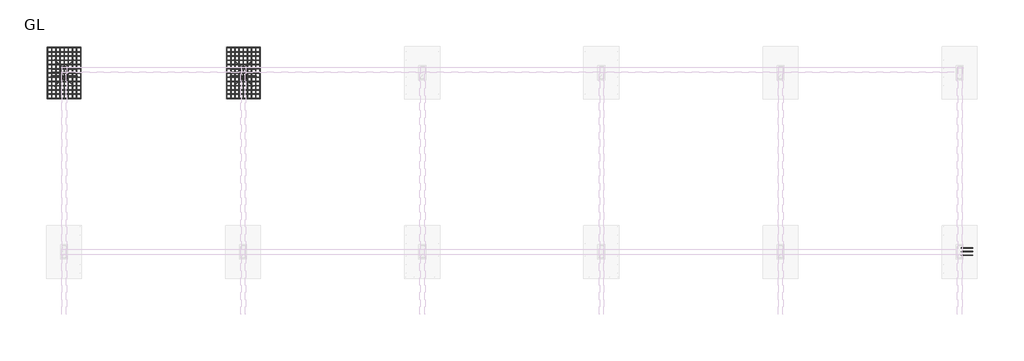
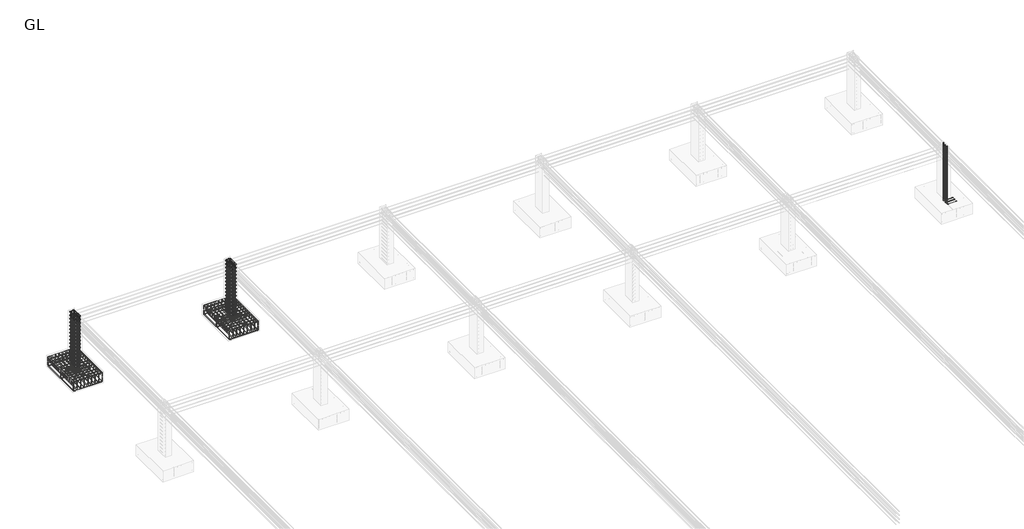
# One storey, part 14 of 16: 23 reinforcing bars.
"""IFC4 building model written with IfcOpenShell, lengths in millimetres."""

from ifc_helpers import new_model, si_unit, point, frame, origin, place, context, project, spatial, polyline, circle_curve, trimmed, segment, composite_curve, source, transform, mapped, element, save
from ifc_brep_helpers import swept_disk

model = new_model("IFC4")

# Units and contexts
model_context = context("Model", 3, world=origin())
ifc_project = project(units=[si_unit("LENGTHUNIT", "METRE", prefix="MILLI")], contexts=[model_context])

# Site, building, storey
site = spatial("IfcSite", under=ifc_project)
building = spatial("IfcBuilding", under=site)
storey = spatial("IfcBuildingStorey", under=building, Name="GL", Elevation=-1829.0)

# Reinforcing bars
placement = place(None, origin())
reinforcing_bar_shape = source(origin(), model_context, "Body", "SolidModel", [
    swept_disk(composite_curve([segment(polyline([(-22242.9544379, 4968.8832479, -2089.0), (-22242.9544379, 4968.8832479, -2213.0)]), True, "CONTINUOUS"), segment(trimmed(circle_curve(frame((-22272.9544379, 4968.8832479, -2213.0), z_axis=(0.0, 1.0, 0.0), x_axis=(30.0, 0.0, 0.0)), 30.0), [point((-22242.9544379, 4968.8832479, -2213.0))], [point((-22272.9544379, 4968.8832479, -2243.0))], True, "CARTESIAN"), True, "CONTINUOUS"), segment(polyline([(-22272.9544379, 4968.8832479, -2243.0), (-23340.9544379, 4968.8832479, -2243.0)]), True, "CONTINUOUS"), segment(trimmed(circle_curve(frame((-23340.9544379, 4968.8832479, -2213.0), z_axis=(0.0, 1.0, 0.0), x_axis=(0.0, 0.0, -30.0)), 30.0), [point((-23340.9544379, 4968.8832479, -2243.0))], [point((-23370.9544379, 4968.8832479, -2213.0))], True, "CARTESIAN"), True, "CONTINUOUS"), segment(polyline([(-23370.9544379, 4968.8832479, -2213.0), (-23370.9544379, 4968.8832479, -2089.0)]), True, "CONTINUOUS")], self_intersect=False), 6.0),
])
element("IfcReinforcingBar", 1, at=placement, inside=storey, context=model_context, shape_type="MappedRepresentation", body=[
    mapped(reinforcing_bar_shape, transform((0.0, 0.0, 0.0), x_axis=(1.0, 0.0, 0.0), y_axis=(0.0, 1.0, 0.0), z_axis=(0.0, 0.0, 1.0))),
    mapped(reinforcing_bar_shape, transform((0.0, -864.0, 0.0), x_axis=(1.0, 0.0, 0.0), y_axis=(0.0, 1.0, 0.0), z_axis=(0.0, 0.0, 1.0))),
    mapped(reinforcing_bar_shape, transform((0.0, -1728.0, 0.0), x_axis=(1.0, 0.0, 0.0), y_axis=(0.0, 1.0, 0.0), z_axis=(0.0, 0.0, 1.0))),
])
reinforcing_bar_2_shape = source(origin(), model_context, "Body", "SolidModel", [
    swept_disk(composite_curve([segment(polyline([(-23370.9544379, 4968.8832479, -2022.436678), (-23370.9544379, 4968.8832479, -1898.436678)]), True, "CONTINUOUS"), segment(trimmed(circle_curve(frame((-23340.9544379, 4968.8832479, -1898.436678), z_axis=(0.0, 1.0, 0.0), x_axis=(-30.0, 0.0, 0.0)), 30.0), [point((-23370.9544379, 4968.8832479, -1898.436678))], [point((-23340.9544379, 4968.8832479, -1868.436678))], True, "CARTESIAN"), True, "CONTINUOUS"), segment(polyline([(-23340.9544379, 4968.8832479, -1868.436678), (-22272.9544379, 4968.8832479, -1868.436678)]), True, "CONTINUOUS"), segment(trimmed(circle_curve(frame((-22272.9544379, 4968.8832479, -1898.436678), z_axis=(0.0, 1.0, 0.0), x_axis=(0.0, 0.0, 30.0)), 30.0), [point((-22272.9544379, 4968.8832479, -1868.436678))], [point((-22242.9544379, 4968.8832479, -1898.436678))], True, "CARTESIAN"), True, "CONTINUOUS"), segment(polyline([(-22242.9544379, 4968.8832479, -1898.436678), (-22242.9544379, 4968.8832479, -2022.436678)]), True, "CONTINUOUS")], self_intersect=False), 6.0),
])
element("IfcReinforcingBar", 2, at=placement, inside=storey, context=model_context, shape_type="MappedRepresentation", body=[
    mapped(reinforcing_bar_2_shape, transform((0.0, 0.0, 0.0), x_axis=(1.0, 0.0, 0.0), y_axis=(0.0, 1.0, 0.0), z_axis=(0.0, 0.0, 1.0))),
    mapped(reinforcing_bar_2_shape, transform((0.0, -144.0, 0.0), x_axis=(1.0, 0.0, 0.0), y_axis=(0.0, 1.0, 0.0), z_axis=(0.0, 0.0, 1.0))),
    mapped(reinforcing_bar_2_shape, transform((0.0, -288.0, 0.0), x_axis=(1.0, 0.0, 0.0), y_axis=(0.0, 1.0, 0.0), z_axis=(0.0, 0.0, 1.0))),
    mapped(reinforcing_bar_2_shape, transform((0.0, -432.0, 0.0), x_axis=(1.0, 0.0, 0.0), y_axis=(0.0, 1.0, 0.0), z_axis=(0.0, 0.0, 1.0))),
    mapped(reinforcing_bar_2_shape, transform((0.0, -576.0, 0.0), x_axis=(1.0, 0.0, 0.0), y_axis=(0.0, 1.0, 0.0), z_axis=(0.0, 0.0, 1.0))),
    mapped(reinforcing_bar_2_shape, transform((0.0, -720.0, 0.0), x_axis=(1.0, 0.0, 0.0), y_axis=(0.0, 1.0, 0.0), z_axis=(0.0, 0.0, 1.0))),
    mapped(reinforcing_bar_2_shape, transform((0.0, -864.0, 0.0), x_axis=(1.0, 0.0, 0.0), y_axis=(0.0, 1.0, 0.0), z_axis=(0.0, 0.0, 1.0))),
    mapped(reinforcing_bar_2_shape, transform((0.0, -1008.0, 0.0), x_axis=(1.0, 0.0, 0.0), y_axis=(0.0, 1.0, 0.0), z_axis=(0.0, 0.0, 1.0))),
    mapped(reinforcing_bar_2_shape, transform((0.0, -1152.0, 0.0), x_axis=(1.0, 0.0, 0.0), y_axis=(0.0, 1.0, 0.0), z_axis=(0.0, 0.0, 1.0))),
    mapped(reinforcing_bar_2_shape, transform((0.0, -1296.0, 0.0), x_axis=(1.0, 0.0, 0.0), y_axis=(0.0, 1.0, 0.0), z_axis=(0.0, 0.0, 1.0))),
    mapped(reinforcing_bar_2_shape, transform((0.0, -1440.0, 0.0), x_axis=(1.0, 0.0, 0.0), y_axis=(0.0, 1.0, 0.0), z_axis=(0.0, 0.0, 1.0))),
    mapped(reinforcing_bar_2_shape, transform((0.0, -1584.0, 0.0), x_axis=(1.0, 0.0, 0.0), y_axis=(0.0, 1.0, 0.0), z_axis=(0.0, 0.0, 1.0))),
    mapped(reinforcing_bar_2_shape, transform((0.0, -1728.0, 0.0), x_axis=(1.0, 0.0, 0.0), y_axis=(0.0, 1.0, 0.0), z_axis=(0.0, 0.0, 1.0))),
])
reinforcing_bar_3_shape = source(origin(), model_context, "Body", "SolidModel", [
    swept_disk(composite_curve([segment(polyline([(-23370.9544379, 3240.8832479, -2027.5081232), (-23370.9544379, 3240.8832479, -1903.5081232)]), True, "CONTINUOUS"), segment(trimmed(circle_curve(frame((-23370.9544379, 3270.8832479, -1903.5081232), z_axis=(-1.0, 0.0, 0.0), x_axis=(0.0, -30.0, 0.0)), 30.0), [point((-23370.9544379, 3240.8832479, -1903.5081232))], [point((-23370.9544379, 3270.8832479, -1873.5081232))], True, "CARTESIAN"), True, "CONTINUOUS"), segment(polyline([(-23370.9544379, 3270.8832479, -1873.5081232), (-23370.9544379, 4938.8832479, -1873.5081232)]), True, "CONTINUOUS"), segment(trimmed(circle_curve(frame((-23370.9544379, 4938.8832479, -1903.5081232), z_axis=(-1.0, 0.0, 0.0), x_axis=(0.0, 0.0, 30.0)), 30.0), [point((-23370.9544379, 4938.8832479, -1873.5081232))], [point((-23370.9544379, 4968.8832479, -1903.5081232))], True, "CARTESIAN"), True, "CONTINUOUS"), segment(polyline([(-23370.9544379, 4968.8832479, -1903.5081232), (-23370.9544379, 4968.8832479, -2027.5081232)]), True, "CONTINUOUS")], self_intersect=False), 6.0),
])
element("IfcReinforcingBar", 3, at=placement, inside=storey, context=model_context, shape_type="MappedRepresentation", body=[
    mapped(reinforcing_bar_3_shape, transform((0.0, 0.0, 0.0), x_axis=(1.0, 0.0, 0.0), y_axis=(0.0, 1.0, 0.0), z_axis=(0.0, 0.0, 1.0))),
    mapped(reinforcing_bar_3_shape, transform((141.0, 0.0, 0.0), x_axis=(1.0, 0.0, 0.0), y_axis=(0.0, 1.0, 0.0), z_axis=(0.0, 0.0, 1.0))),
    mapped(reinforcing_bar_3_shape, transform((282.0, 0.0, 0.0), x_axis=(1.0, 0.0, 0.0), y_axis=(0.0, 1.0, 0.0), z_axis=(0.0, 0.0, 1.0))),
    mapped(reinforcing_bar_3_shape, transform((423.0, 0.0, 0.0), x_axis=(1.0, 0.0, 0.0), y_axis=(0.0, 1.0, 0.0), z_axis=(0.0, 0.0, 1.0))),
    mapped(reinforcing_bar_3_shape, transform((564.0, 0.0, 0.0), x_axis=(1.0, 0.0, 0.0), y_axis=(0.0, 1.0, 0.0), z_axis=(0.0, 0.0, 1.0))),
    mapped(reinforcing_bar_3_shape, transform((705.0, 0.0, 0.0), x_axis=(1.0, 0.0, 0.0), y_axis=(0.0, 1.0, 0.0), z_axis=(0.0, 0.0, 1.0))),
    mapped(reinforcing_bar_3_shape, transform((846.0, 0.0, 0.0), x_axis=(1.0, 0.0, 0.0), y_axis=(0.0, 1.0, 0.0), z_axis=(0.0, 0.0, 1.0))),
    mapped(reinforcing_bar_3_shape, transform((987.0, 0.0, 0.0), x_axis=(1.0, 0.0, 0.0), y_axis=(0.0, 1.0, 0.0), z_axis=(0.0, 0.0, 1.0))),
    mapped(reinforcing_bar_3_shape, transform((1128.0, 0.0, 0.0), x_axis=(1.0, 0.0, 0.0), y_axis=(0.0, 1.0, 0.0), z_axis=(0.0, 0.0, 1.0))),
])
reinforcing_bar_4_shape = source(origin(), model_context, "Body", "SolidModel", [
    swept_disk(composite_curve([segment(polyline([(-22242.9544379, 3240.8832479, -2080.6239909), (-22242.9544379, 3240.8832479, -2204.6239909)]), True, "CONTINUOUS"), segment(trimmed(circle_curve(frame((-22242.9544379, 3270.8832479, -2204.6239909), z_axis=(1.0, 0.0, 0.0), x_axis=(0.0, -30.0, 0.0)), 30.0), [point((-22242.9544379, 3240.8832479, -2204.6239909))], [point((-22242.9544379, 3270.8832479, -2234.6239909))], True, "CARTESIAN"), True, "CONTINUOUS"), segment(polyline([(-22242.9544379, 3270.8832479, -2234.6239909), (-22242.9544379, 4925.8578108, -2234.6239909)]), True, "CONTINUOUS"), segment(trimmed(circle_curve(frame((-22242.9544379, 4925.8578108, -2204.6239909), z_axis=(1.0, 0.0, 0.0), x_axis=(0.0, 0.0, -30.0)), 30.0), [point((-22242.9544379, 4925.8578108, -2234.6239909))], [point((-22242.9544379, 4955.8578108, -2204.6239909))], True, "CARTESIAN"), True, "CONTINUOUS"), segment(polyline([(-22242.9544379, 4955.8578108, -2204.6239909), (-22242.9544379, 4955.8578108, -2080.6239909)]), True, "CONTINUOUS")], self_intersect=False), 6.0),
])
element("IfcReinforcingBar", 4, at=placement, inside=storey, context=model_context, shape_type="MappedRepresentation", body=[
    mapped(reinforcing_bar_4_shape, transform((0.0, 0.0, 0.0), x_axis=(1.0, 0.0, 0.0), y_axis=(0.0, 1.0, 0.0), z_axis=(0.0, 0.0, 1.0))),
    mapped(reinforcing_bar_4_shape, transform((-141.0, 0.0, 0.0), x_axis=(1.0, 0.0, 0.0), y_axis=(0.0, 1.0, 0.0), z_axis=(0.0, 0.0, 1.0))),
    mapped(reinforcing_bar_4_shape, transform((-282.0, 0.0, 0.0), x_axis=(1.0, 0.0, 0.0), y_axis=(0.0, 1.0, 0.0), z_axis=(0.0, 0.0, 1.0))),
    mapped(reinforcing_bar_4_shape, transform((-423.0, 0.0, 0.0), x_axis=(1.0, 0.0, 0.0), y_axis=(0.0, 1.0, 0.0), z_axis=(0.0, 0.0, 1.0))),
    mapped(reinforcing_bar_4_shape, transform((-564.0, 0.0, 0.0), x_axis=(1.0, 0.0, 0.0), y_axis=(0.0, 1.0, 0.0), z_axis=(0.0, 0.0, 1.0))),
    mapped(reinforcing_bar_4_shape, transform((-705.0, 0.0, 0.0), x_axis=(1.0, 0.0, 0.0), y_axis=(0.0, 1.0, 0.0), z_axis=(0.0, 0.0, 1.0))),
    mapped(reinforcing_bar_4_shape, transform((-846.0, 0.0, 0.0), x_axis=(1.0, 0.0, 0.0), y_axis=(0.0, 1.0, 0.0), z_axis=(0.0, 0.0, 1.0))),
    mapped(reinforcing_bar_4_shape, transform((-987.0, 0.0, 0.0), x_axis=(1.0, 0.0, 0.0), y_axis=(0.0, 1.0, 0.0), z_axis=(0.0, 0.0, 1.0))),
    mapped(reinforcing_bar_4_shape, transform((-1128.0, 0.0, 0.0), x_axis=(1.0, 0.0, 0.0), y_axis=(0.0, 1.0, 0.0), z_axis=(0.0, 0.0, 1.0))),
])
reinforcing_bar_5_shape = source(origin(), model_context, "Body", "SolidModel", [
    swept_disk(composite_curve([segment(polyline([(-16146.9544379, 4968.8832479, -2089.0), (-16146.9544379, 4968.8832479, -2213.0)]), True, "CONTINUOUS"), segment(trimmed(circle_curve(frame((-16176.9544379, 4968.8832479, -2213.0), z_axis=(0.0, 1.0, 0.0), x_axis=(30.0, 0.0, 0.0)), 30.0), [point((-16146.9544379, 4968.8832479, -2213.0))], [point((-16176.9544379, 4968.8832479, -2243.0))], True, "CARTESIAN"), True, "CONTINUOUS"), segment(polyline([(-16176.9544379, 4968.8832479, -2243.0), (-17244.9544379, 4968.8832479, -2243.0)]), True, "CONTINUOUS"), segment(trimmed(circle_curve(frame((-17244.9544379, 4968.8832479, -2213.0), z_axis=(0.0, 1.0, 0.0), x_axis=(0.0, 0.0, -30.0)), 30.0), [point((-17244.9544379, 4968.8832479, -2243.0))], [point((-17274.9544379, 4968.8832479, -2213.0))], True, "CARTESIAN"), True, "CONTINUOUS"), segment(polyline([(-17274.9544379, 4968.8832479, -2213.0), (-17274.9544379, 4968.8832479, -2089.0)]), True, "CONTINUOUS")], self_intersect=False), 6.0),
])
element("IfcReinforcingBar", 5, at=placement, inside=storey, context=model_context, shape_type="MappedRepresentation", body=[
    mapped(reinforcing_bar_5_shape, transform((0.0, 0.0, 0.0), x_axis=(1.0, 0.0, 0.0), y_axis=(0.0, 1.0, 0.0), z_axis=(0.0, 0.0, 1.0))),
    mapped(reinforcing_bar_5_shape, transform((0.0, -864.0, 0.0), x_axis=(1.0, 0.0, 0.0), y_axis=(0.0, 1.0, 0.0), z_axis=(0.0, 0.0, 1.0))),
    mapped(reinforcing_bar_5_shape, transform((0.0, -1728.0, 0.0), x_axis=(1.0, 0.0, 0.0), y_axis=(0.0, 1.0, 0.0), z_axis=(0.0, 0.0, 1.0))),
])
reinforcing_bar_6_shape = source(origin(), model_context, "Body", "SolidModel", [
    swept_disk(composite_curve([segment(polyline([(-17274.9544379, 4968.8832479, -2022.436678), (-17274.9544379, 4968.8832479, -1898.436678)]), True, "CONTINUOUS"), segment(trimmed(circle_curve(frame((-17244.9544379, 4968.8832479, -1898.436678), z_axis=(0.0, 1.0, 0.0), x_axis=(-30.0, 0.0, 0.0)), 30.0), [point((-17274.9544379, 4968.8832479, -1898.436678))], [point((-17244.9544379, 4968.8832479, -1868.436678))], True, "CARTESIAN"), True, "CONTINUOUS"), segment(polyline([(-17244.9544379, 4968.8832479, -1868.436678), (-16176.9544379, 4968.8832479, -1868.436678)]), True, "CONTINUOUS"), segment(trimmed(circle_curve(frame((-16176.9544379, 4968.8832479, -1898.436678), z_axis=(0.0, 1.0, 0.0), x_axis=(0.0, 0.0, 30.0)), 30.0), [point((-16176.9544379, 4968.8832479, -1868.436678))], [point((-16146.9544379, 4968.8832479, -1898.436678))], True, "CARTESIAN"), True, "CONTINUOUS"), segment(polyline([(-16146.9544379, 4968.8832479, -1898.436678), (-16146.9544379, 4968.8832479, -2022.436678)]), True, "CONTINUOUS")], self_intersect=False), 6.0),
])
element("IfcReinforcingBar", 6, at=placement, inside=storey, context=model_context, shape_type="MappedRepresentation", body=[
    mapped(reinforcing_bar_6_shape, transform((0.0, 0.0, 0.0), x_axis=(1.0, 0.0, 0.0), y_axis=(0.0, 1.0, 0.0), z_axis=(0.0, 0.0, 1.0))),
    mapped(reinforcing_bar_6_shape, transform((0.0, -144.0, 0.0), x_axis=(1.0, 0.0, 0.0), y_axis=(0.0, 1.0, 0.0), z_axis=(0.0, 0.0, 1.0))),
    mapped(reinforcing_bar_6_shape, transform((0.0, -288.0, 0.0), x_axis=(1.0, 0.0, 0.0), y_axis=(0.0, 1.0, 0.0), z_axis=(0.0, 0.0, 1.0))),
    mapped(reinforcing_bar_6_shape, transform((0.0, -432.0, 0.0), x_axis=(1.0, 0.0, 0.0), y_axis=(0.0, 1.0, 0.0), z_axis=(0.0, 0.0, 1.0))),
    mapped(reinforcing_bar_6_shape, transform((0.0, -576.0, 0.0), x_axis=(1.0, 0.0, 0.0), y_axis=(0.0, 1.0, 0.0), z_axis=(0.0, 0.0, 1.0))),
    mapped(reinforcing_bar_6_shape, transform((0.0, -720.0, 0.0), x_axis=(1.0, 0.0, 0.0), y_axis=(0.0, 1.0, 0.0), z_axis=(0.0, 0.0, 1.0))),
    mapped(reinforcing_bar_6_shape, transform((0.0, -864.0, 0.0), x_axis=(1.0, 0.0, 0.0), y_axis=(0.0, 1.0, 0.0), z_axis=(0.0, 0.0, 1.0))),
    mapped(reinforcing_bar_6_shape, transform((0.0, -1008.0, 0.0), x_axis=(1.0, 0.0, 0.0), y_axis=(0.0, 1.0, 0.0), z_axis=(0.0, 0.0, 1.0))),
    mapped(reinforcing_bar_6_shape, transform((0.0, -1152.0, 0.0), x_axis=(1.0, 0.0, 0.0), y_axis=(0.0, 1.0, 0.0), z_axis=(0.0, 0.0, 1.0))),
    mapped(reinforcing_bar_6_shape, transform((0.0, -1296.0, 0.0), x_axis=(1.0, 0.0, 0.0), y_axis=(0.0, 1.0, 0.0), z_axis=(0.0, 0.0, 1.0))),
    mapped(reinforcing_bar_6_shape, transform((0.0, -1440.0, 0.0), x_axis=(1.0, 0.0, 0.0), y_axis=(0.0, 1.0, 0.0), z_axis=(0.0, 0.0, 1.0))),
    mapped(reinforcing_bar_6_shape, transform((0.0, -1584.0, 0.0), x_axis=(1.0, 0.0, 0.0), y_axis=(0.0, 1.0, 0.0), z_axis=(0.0, 0.0, 1.0))),
    mapped(reinforcing_bar_6_shape, transform((0.0, -1728.0, 0.0), x_axis=(1.0, 0.0, 0.0), y_axis=(0.0, 1.0, 0.0), z_axis=(0.0, 0.0, 1.0))),
])
reinforcing_bar_7_shape = source(origin(), model_context, "Body", "SolidModel", [
    swept_disk(composite_curve([segment(polyline([(-17274.9544379, 3240.8832479, -2027.5081232), (-17274.9544379, 3240.8832479, -1903.5081232)]), True, "CONTINUOUS"), segment(trimmed(circle_curve(frame((-17274.9544379, 3270.8832479, -1903.5081232), z_axis=(-1.0, 0.0, 0.0), x_axis=(0.0, -30.0, 0.0)), 30.0), [point((-17274.9544379, 3240.8832479, -1903.5081232))], [point((-17274.9544379, 3270.8832479, -1873.5081232))], True, "CARTESIAN"), True, "CONTINUOUS"), segment(polyline([(-17274.9544379, 3270.8832479, -1873.5081232), (-17274.9544379, 4938.8832479, -1873.5081232)]), True, "CONTINUOUS"), segment(trimmed(circle_curve(frame((-17274.9544379, 4938.8832479, -1903.5081232), z_axis=(-1.0, 0.0, 0.0), x_axis=(0.0, 0.0, 30.0)), 30.0), [point((-17274.9544379, 4938.8832479, -1873.5081232))], [point((-17274.9544379, 4968.8832479, -1903.5081232))], True, "CARTESIAN"), True, "CONTINUOUS"), segment(polyline([(-17274.9544379, 4968.8832479, -1903.5081232), (-17274.9544379, 4968.8832479, -2027.5081232)]), True, "CONTINUOUS")], self_intersect=False), 6.0),
])
element("IfcReinforcingBar", 7, at=placement, inside=storey, context=model_context, shape_type="MappedRepresentation", body=[
    mapped(reinforcing_bar_7_shape, transform((0.0, 0.0, 0.0), x_axis=(1.0, 0.0, 0.0), y_axis=(0.0, 1.0, 0.0), z_axis=(0.0, 0.0, 1.0))),
    mapped(reinforcing_bar_7_shape, transform((141.0, 0.0, 0.0), x_axis=(1.0, 0.0, 0.0), y_axis=(0.0, 1.0, 0.0), z_axis=(0.0, 0.0, 1.0))),
    mapped(reinforcing_bar_7_shape, transform((282.0, 0.0, 0.0), x_axis=(1.0, 0.0, 0.0), y_axis=(0.0, 1.0, 0.0), z_axis=(0.0, 0.0, 1.0))),
    mapped(reinforcing_bar_7_shape, transform((423.0, 0.0, 0.0), x_axis=(1.0, 0.0, 0.0), y_axis=(0.0, 1.0, 0.0), z_axis=(0.0, 0.0, 1.0))),
    mapped(reinforcing_bar_7_shape, transform((564.0, 0.0, 0.0), x_axis=(1.0, 0.0, 0.0), y_axis=(0.0, 1.0, 0.0), z_axis=(0.0, 0.0, 1.0))),
    mapped(reinforcing_bar_7_shape, transform((705.0, 0.0, 0.0), x_axis=(1.0, 0.0, 0.0), y_axis=(0.0, 1.0, 0.0), z_axis=(0.0, 0.0, 1.0))),
    mapped(reinforcing_bar_7_shape, transform((846.0, 0.0, 0.0), x_axis=(1.0, 0.0, 0.0), y_axis=(0.0, 1.0, 0.0), z_axis=(0.0, 0.0, 1.0))),
    mapped(reinforcing_bar_7_shape, transform((987.0, 0.0, 0.0), x_axis=(1.0, 0.0, 0.0), y_axis=(0.0, 1.0, 0.0), z_axis=(0.0, 0.0, 1.0))),
    mapped(reinforcing_bar_7_shape, transform((1128.0, 0.0, 0.0), x_axis=(1.0, 0.0, 0.0), y_axis=(0.0, 1.0, 0.0), z_axis=(0.0, 0.0, 1.0))),
])
reinforcing_bar_8_shape = source(origin(), model_context, "Body", "SolidModel", [
    swept_disk(composite_curve([segment(polyline([(-16146.9544379, 3240.8832479, -2080.6239909), (-16146.9544379, 3240.8832479, -2204.6239909)]), True, "CONTINUOUS"), segment(trimmed(circle_curve(frame((-16146.9544379, 3270.8832479, -2204.6239909), z_axis=(1.0, 0.0, 0.0), x_axis=(0.0, -30.0, 0.0)), 30.0), [point((-16146.9544379, 3240.8832479, -2204.6239909))], [point((-16146.9544379, 3270.8832479, -2234.6239909))], True, "CARTESIAN"), True, "CONTINUOUS"), segment(polyline([(-16146.9544379, 3270.8832479, -2234.6239909), (-16146.9544379, 4925.8578108, -2234.6239909)]), True, "CONTINUOUS"), segment(trimmed(circle_curve(frame((-16146.9544379, 4925.8578108, -2204.6239909), z_axis=(1.0, 0.0, 0.0), x_axis=(0.0, 0.0, -30.0)), 30.0), [point((-16146.9544379, 4925.8578108, -2234.6239909))], [point((-16146.9544379, 4955.8578108, -2204.6239909))], True, "CARTESIAN"), True, "CONTINUOUS"), segment(polyline([(-16146.9544379, 4955.8578108, -2204.6239909), (-16146.9544379, 4955.8578108, -2080.6239909)]), True, "CONTINUOUS")], self_intersect=False), 6.0),
])
element("IfcReinforcingBar", 8, at=placement, inside=storey, context=model_context, shape_type="MappedRepresentation", body=[
    mapped(reinforcing_bar_8_shape, transform((0.0, 0.0, 0.0), x_axis=(1.0, 0.0, 0.0), y_axis=(0.0, 1.0, 0.0), z_axis=(0.0, 0.0, 1.0))),
    mapped(reinforcing_bar_8_shape, transform((-141.0, 0.0, 0.0), x_axis=(1.0, 0.0, 0.0), y_axis=(0.0, 1.0, 0.0), z_axis=(0.0, 0.0, 1.0))),
    mapped(reinforcing_bar_8_shape, transform((-282.0, 0.0, 0.0), x_axis=(1.0, 0.0, 0.0), y_axis=(0.0, 1.0, 0.0), z_axis=(0.0, 0.0, 1.0))),
    mapped(reinforcing_bar_8_shape, transform((-423.0, 0.0, 0.0), x_axis=(1.0, 0.0, 0.0), y_axis=(0.0, 1.0, 0.0), z_axis=(0.0, 0.0, 1.0))),
    mapped(reinforcing_bar_8_shape, transform((-564.0, 0.0, 0.0), x_axis=(1.0, 0.0, 0.0), y_axis=(0.0, 1.0, 0.0), z_axis=(0.0, 0.0, 1.0))),
    mapped(reinforcing_bar_8_shape, transform((-705.0, 0.0, 0.0), x_axis=(1.0, 0.0, 0.0), y_axis=(0.0, 1.0, 0.0), z_axis=(0.0, 0.0, 1.0))),
    mapped(reinforcing_bar_8_shape, transform((-846.0, 0.0, 0.0), x_axis=(1.0, 0.0, 0.0), y_axis=(0.0, 1.0, 0.0), z_axis=(0.0, 0.0, 1.0))),
    mapped(reinforcing_bar_8_shape, transform((-987.0, 0.0, 0.0), x_axis=(1.0, 0.0, 0.0), y_axis=(0.0, 1.0, 0.0), z_axis=(0.0, 0.0, 1.0))),
    mapped(reinforcing_bar_8_shape, transform((-1128.0, 0.0, 0.0), x_axis=(1.0, 0.0, 0.0), y_axis=(0.0, 1.0, 0.0), z_axis=(0.0, 0.0, 1.0))),
])
reinforcing_bar_9_shape = source(origin(), model_context, "Body", "SolidModel", [
    swept_disk(composite_curve([segment(polyline([(-16703.4864005, 4029.7776922, -1793.0), (-16791.1676414, 3942.0964514, -1793.0)]), True, "CONTINUOUS"), segment(trimmed(circle_curve(frame((-16769.9544379, 3920.8832479, -1793.0), z_axis=(0.0, 0.0, 1.0), x_axis=(-21.21320349999951, 21.213203500000418, 0.0)), 30.0), [point((-16791.1676414, 3942.0964514, -1793.0))], [point((-16769.9544379, 3890.8832479, -1793.0))], True, "CARTESIAN"), True, "CONTINUOUS"), segment(polyline([(-16769.9544379, 3890.8832479, -1793.0), (-16651.9544379, 3890.8832479, -1793.0)]), True, "CONTINUOUS"), segment(trimmed(circle_curve(frame((-16651.9544379, 3920.8832479, -1793.0), z_axis=(0.0, 0.0, 1.0), x_axis=(0.0, -30.0, 0.0)), 30.0), [point((-16651.9544379, 3890.8832479, -1793.0))], [point((-16621.9544379, 3920.8832479, -1793.0))], True, "CARTESIAN"), True, "CONTINUOUS"), segment(polyline([(-16621.9544379, 3920.8832479, -1793.0), (-16621.9544379, 4288.8832479, -1793.0)]), True, "CONTINUOUS"), segment(trimmed(circle_curve(frame((-16651.8864962, 4288.8832479, -1795.0178916), z_axis=(-0.06726305234213417, 0.0, 0.9977352764083365), x_axis=(29.93205830000079, 0.0, 2.0178915999999845)), 30.0), [point((-16621.9544379, 4288.8832479, -1793.0))], [point((-16651.8864962, 4318.8832479, -1795.0178916))], True, "CARTESIAN"), True, "CONTINUOUS"), segment(polyline([(-16651.8864962, 4318.8832479, -1795.0178916), (-16770.0223796, 4318.8832479, -1802.9821084)]), True, "CONTINUOUS"), segment(trimmed(circle_curve(frame((-16770.0223796, 4288.8832479, -1802.9821084), z_axis=(-0.06726305234213417, 0.0, 0.9977352764083365), x_axis=(0.0, 30.0, 0.0)), 30.0), [point((-16770.0223796, 4318.8832479, -1802.9821084))], [point((-16799.9544379, 4288.8832479, -1805.0))], True, "CARTESIAN"), True, "CONTINUOUS"), segment(polyline([(-16799.9544379, 4288.8832479, -1805.0), (-16799.9544379, 3920.8832479, -1805.0)]), True, "CONTINUOUS"), segment(trimmed(circle_curve(frame((-16769.9544379, 3920.8832479, -1805.0), z_axis=(0.0, 0.0, 1.0), x_axis=(-30.0, 0.0, 0.0)), 30.0), [point((-16799.9544379, 3920.8832479, -1805.0))], [point((-16748.7412345, 3899.6700445, -1805.0))], True, "CARTESIAN"), True, "CONTINUOUS"), segment(polyline([(-16748.7412345, 3899.6700445, -1805.0), (-16661.0599936, 3987.3512854, -1805.0)]), True, "CONTINUOUS")], self_intersect=False), 6.0),
])
element("IfcReinforcingBar", 9, at=placement, inside=storey, context=model_context, shape_type="MappedRepresentation", body=[
    mapped(reinforcing_bar_9_shape, transform((0.0, 0.0, 0.0), x_axis=(1.0, 0.0, 0.0), y_axis=(0.0, 1.0, 0.0), z_axis=(0.0, 0.0, 1.0))),
    mapped(reinforcing_bar_9_shape, transform((0.0, 0.0, 144.8571429), x_axis=(1.0, 0.0, 0.0), y_axis=(0.0, 1.0, 0.0), z_axis=(0.0, 0.0, 1.0))),
    mapped(reinforcing_bar_9_shape, transform((0.0, 0.0, 289.7142857), x_axis=(1.0, 0.0, 0.0), y_axis=(0.0, 1.0, 0.0), z_axis=(0.0, 0.0, 1.0))),
    mapped(reinforcing_bar_9_shape, transform((0.0, 0.0, 434.5714286), x_axis=(1.0, 0.0, 0.0), y_axis=(0.0, 1.0, 0.0), z_axis=(0.0, 0.0, 1.0))),
    mapped(reinforcing_bar_9_shape, transform((0.0, 0.0, 579.4285714), x_axis=(1.0, 0.0, 0.0), y_axis=(0.0, 1.0, 0.0), z_axis=(0.0, 0.0, 1.0))),
    mapped(reinforcing_bar_9_shape, transform((0.0, 0.0, 724.2857143), x_axis=(1.0, 0.0, 0.0), y_axis=(0.0, 1.0, 0.0), z_axis=(0.0, 0.0, 1.0))),
    mapped(reinforcing_bar_9_shape, transform((0.0, 0.0, 869.1428571), x_axis=(1.0, 0.0, 0.0), y_axis=(0.0, 1.0, 0.0), z_axis=(0.0, 0.0, 1.0))),
    mapped(reinforcing_bar_9_shape, transform((0.0, 0.0, 1014.0), x_axis=(1.0, 0.0, 0.0), y_axis=(0.0, 1.0, 0.0), z_axis=(0.0, 0.0, 1.0))),
    mapped(reinforcing_bar_9_shape, transform((0.0, 0.0, 1158.8571429), x_axis=(1.0, 0.0, 0.0), y_axis=(0.0, 1.0, 0.0), z_axis=(0.0, 0.0, 1.0))),
    mapped(reinforcing_bar_9_shape, transform((0.0, 0.0, 1303.7142857), x_axis=(1.0, 0.0, 0.0), y_axis=(0.0, 1.0, 0.0), z_axis=(0.0, 0.0, 1.0))),
    mapped(reinforcing_bar_9_shape, transform((0.0, 0.0, 1448.5714286), x_axis=(1.0, 0.0, 0.0), y_axis=(0.0, 1.0, 0.0), z_axis=(0.0, 0.0, 1.0))),
    mapped(reinforcing_bar_9_shape, transform((0.0, 0.0, 1593.4285714), x_axis=(1.0, 0.0, 0.0), y_axis=(0.0, 1.0, 0.0), z_axis=(0.0, 0.0, 1.0))),
    mapped(reinforcing_bar_9_shape, transform((0.0, 0.0, 1738.2857143), x_axis=(1.0, 0.0, 0.0), y_axis=(0.0, 1.0, 0.0), z_axis=(0.0, 0.0, 1.0))),
    mapped(reinforcing_bar_9_shape, transform((0.0, 0.0, 1883.1428571), x_axis=(1.0, 0.0, 0.0), y_axis=(0.0, 1.0, 0.0), z_axis=(0.0, 0.0, 1.0))),
    mapped(reinforcing_bar_9_shape, transform((0.0, 0.0, 2028.0), x_axis=(1.0, 0.0, 0.0), y_axis=(0.0, 1.0, 0.0), z_axis=(0.0, 0.0, 1.0))),
])
element("IfcReinforcingBar", 10, at=placement, inside=storey, context=model_context, shape_type="SolidModel", body=[
    swept_disk(composite_curve([segment(polyline([(-16768.0642232, 3919.9357561, 241.0), (-16768.0642232, 3919.9357561, -2129.0)]), True, "CONTINUOUS"), segment(trimmed(circle_curve(frame((-16789.2774266, 3898.7225527, -2129.0), z_axis=(-0.7071067811865187, 0.7071067811865764, 0.0), x_axis=(21.213203400002385, 21.21320340000011, 0.0)), 30.0), [point((-16768.0642232, 3919.9357561, -2129.0))], [point((-16789.2774266, 3898.7225527, -2159.0))], True, "CARTESIAN"), True, "CONTINUOUS"), segment(polyline([(-16789.2774266, 3898.7225527, -2159.0), (-17036.7648, 3651.2351793, -2159.0)]), True, "CONTINUOUS")], self_intersect=False), 6.0),
])
element("IfcReinforcingBar", 11, at=placement, inside=storey, context=model_context, shape_type="SolidModel", body=[
    swept_disk(composite_curve([segment(polyline([(-16768.0642232, 4289.8307397, 241.0), (-16768.0642232, 4289.8307397, -2129.0)]), True, "CONTINUOUS"), segment(trimmed(circle_curve(frame((-16789.2774266, 4311.0439432, -2129.0), z_axis=(0.7071067811865218, 0.7071067811865733, 0.0), x_axis=(21.213203400002385, -21.213203500000418, 0.0)), 30.0), [point((-16768.0642232, 4289.8307397, -2129.0))], [point((-16789.2774266, 4311.0439432, -2159.0))], True, "CARTESIAN"), True, "CONTINUOUS"), segment(polyline([(-16789.2774266, 4311.0439432, -2159.0), (-17036.7648, 4558.5313166, -2159.0)]), True, "CONTINUOUS")], self_intersect=False), 6.0),
])
element("IfcReinforcingBar", 12, at=placement, inside=storey, context=model_context, shape_type="SolidModel", body=[
    swept_disk(composite_curve([segment(polyline([(-16653.8446527, 3919.9357561, 241.0), (-16653.8446527, 3919.9357561, -2129.0)]), True, "CONTINUOUS"), segment(trimmed(circle_curve(frame((-16632.6314492, 3898.7225527, -2129.0), z_axis=(-0.7071067811865248, -0.7071067811865703, 0.0), x_axis=(-21.213203500003146, 21.21320340000011, 0.0)), 30.0), [point((-16653.8446527, 3919.9357561, -2129.0))], [point((-16632.6314492, 3898.7225527, -2159.0))], True, "CARTESIAN"), True, "CONTINUOUS"), segment(polyline([(-16632.6314492, 3898.7225527, -2159.0), (-16385.1440758, 3651.2351793, -2159.0)]), True, "CONTINUOUS")], self_intersect=False), 6.0),
])
element("IfcReinforcingBar", 13, at=placement, inside=storey, context=model_context, shape_type="SolidModel", body=[
    swept_disk(composite_curve([segment(polyline([(-16653.8446527, 4289.8307397, 241.0), (-16653.8446527, 4289.8307397, -2129.0)]), True, "CONTINUOUS"), segment(trimmed(circle_curve(frame((-16632.6314492, 4311.0439432, -2129.0), z_axis=(0.7071067811865157, -0.7071067811865794, 0.0), x_axis=(-21.213203500003146, -21.213203500000418, 0.0)), 30.0), [point((-16653.8446527, 4289.8307397, -2129.0))], [point((-16632.6314492, 4311.0439432, -2159.0))], True, "CARTESIAN"), True, "CONTINUOUS"), segment(polyline([(-16632.6314492, 4311.0439432, -2159.0), (-16385.1440758, 4558.5313166, -2159.0)]), True, "CONTINUOUS")], self_intersect=False), 6.0),
])
reinforcing_bar_10_shape = source(origin(), model_context, "Body", "SolidModel", [
    swept_disk(composite_curve([segment(polyline([(-16768.0642232, 3997.0882595, 241.0), (-16768.0642232, 3997.0882595, -2129.0)]), True, "CONTINUOUS"), segment(trimmed(circle_curve(frame((-16798.0642232, 3997.0882595, -2129.0), z_axis=(0.0, 1.0, 0.0), x_axis=(30.0, 0.0, 0.0)), 30.0), [point((-16768.0642232, 3997.0882595, -2129.0))], [point((-16798.0642232, 3997.0882595, -2159.0))], True, "CARTESIAN"), True, "CONTINUOUS"), segment(polyline([(-16798.0642232, 3997.0882595, -2159.0), (-17148.0642232, 3997.0882595, -2159.0)]), True, "CONTINUOUS")], self_intersect=False), 6.0),
])
element("IfcReinforcingBar", 14, at=placement, inside=storey, context=model_context, shape_type="MappedRepresentation", body=[
    mapped(reinforcing_bar_10_shape, transform((0.0, 0.0, 0.0), x_axis=(1.0, 0.0, 0.0), y_axis=(0.0, 1.0, 0.0), z_axis=(0.0, 0.0, 1.0))),
    mapped(reinforcing_bar_10_shape, transform((0.0, 123.5823926, 0.0), x_axis=(1.0, 0.0, 0.0), y_axis=(0.0, 1.0, 0.0), z_axis=(0.0, 0.0, 1.0))),
    mapped(reinforcing_bar_10_shape, transform((0.0, 247.1647853, 0.0), x_axis=(1.0, 0.0, 0.0), y_axis=(0.0, 1.0, 0.0), z_axis=(0.0, 0.0, 1.0))),
])
reinforcing_bar_11_shape = source(origin(), model_context, "Body", "SolidModel", [
    swept_disk(composite_curve([segment(polyline([(-16653.8446527, 3997.0882595, 241.0), (-16653.8446527, 3997.0882595, -2129.0)]), True, "CONTINUOUS"), segment(trimmed(circle_curve(frame((-16623.8446527, 3997.0882595, -2129.0), z_axis=(0.0, -1.0, 0.0), x_axis=(-30.0, 0.0, 0.0)), 30.0), [point((-16653.8446527, 3997.0882595, -2129.0))], [point((-16623.8446527, 3997.0882595, -2159.0))], True, "CARTESIAN"), True, "CONTINUOUS"), segment(polyline([(-16623.8446527, 3997.0882595, -2159.0), (-16273.8446527, 3997.0882595, -2159.0)]), True, "CONTINUOUS")], self_intersect=False), 6.0),
])
element("IfcReinforcingBar", 15, at=placement, inside=storey, context=model_context, shape_type="MappedRepresentation", body=[
    mapped(reinforcing_bar_11_shape, transform((0.0, 0.0, 0.0), x_axis=(1.0, 0.0, 0.0), y_axis=(0.0, 1.0, 0.0), z_axis=(0.0, 0.0, 1.0))),
    mapped(reinforcing_bar_11_shape, transform((0.0, 123.5823926, 0.0), x_axis=(1.0, 0.0, 0.0), y_axis=(0.0, 1.0, 0.0), z_axis=(0.0, 0.0, 1.0))),
    mapped(reinforcing_bar_11_shape, transform((0.0, 247.1647853, 0.0), x_axis=(1.0, 0.0, 0.0), y_axis=(0.0, 1.0, 0.0), z_axis=(0.0, 0.0, 1.0))),
])
reinforcing_bar_12_shape = source(origin(), model_context, "Body", "SolidModel", [
    swept_disk(composite_curve([segment(polyline([(-22799.4864005, 4029.7776922, -1793.0), (-22887.1676414, 3942.0964514, -1793.0)]), True, "CONTINUOUS"), segment(trimmed(circle_curve(frame((-22865.9544379, 3920.8832479, -1793.0), z_axis=(0.0, 0.0, 1.0), x_axis=(-21.21320349999951, 21.213203500000418, 0.0)), 30.0), [point((-22887.1676414, 3942.0964514, -1793.0))], [point((-22865.9544379, 3890.8832479, -1793.0))], True, "CARTESIAN"), True, "CONTINUOUS"), segment(polyline([(-22865.9544379, 3890.8832479, -1793.0), (-22747.9544379, 3890.8832479, -1793.0)]), True, "CONTINUOUS"), segment(trimmed(circle_curve(frame((-22747.9544379, 3920.8832479, -1793.0), z_axis=(0.0, 0.0, 1.0), x_axis=(0.0, -30.0, 0.0)), 30.0), [point((-22747.9544379, 3890.8832479, -1793.0))], [point((-22717.9544379, 3920.8832479, -1793.0))], True, "CARTESIAN"), True, "CONTINUOUS"), segment(polyline([(-22717.9544379, 3920.8832479, -1793.0), (-22717.9544379, 4288.8832479, -1793.0)]), True, "CONTINUOUS"), segment(trimmed(circle_curve(frame((-22747.8864962, 4288.8832479, -1795.0178916), z_axis=(-0.06726305234213417, 0.0, 0.9977352764083365), x_axis=(29.93205830000079, 0.0, 2.0178915999999845)), 30.0), [point((-22717.9544379, 4288.8832479, -1793.0))], [point((-22747.8864962, 4318.8832479, -1795.0178916))], True, "CARTESIAN"), True, "CONTINUOUS"), segment(polyline([(-22747.8864962, 4318.8832479, -1795.0178916), (-22866.0223796, 4318.8832479, -1802.9821084)]), True, "CONTINUOUS"), segment(trimmed(circle_curve(frame((-22866.0223796, 4288.8832479, -1802.9821084), z_axis=(-0.06726305234213417, 0.0, 0.9977352764083365), x_axis=(0.0, 30.0, 0.0)), 30.0), [point((-22866.0223796, 4318.8832479, -1802.9821084))], [point((-22895.9544379, 4288.8832479, -1805.0))], True, "CARTESIAN"), True, "CONTINUOUS"), segment(polyline([(-22895.9544379, 4288.8832479, -1805.0), (-22895.9544379, 3920.8832479, -1805.0)]), True, "CONTINUOUS"), segment(trimmed(circle_curve(frame((-22865.9544379, 3920.8832479, -1805.0), z_axis=(0.0, 0.0, 1.0), x_axis=(-30.0, 0.0, 0.0)), 30.0), [point((-22895.9544379, 3920.8832479, -1805.0))], [point((-22844.7412345, 3899.6700445, -1805.0))], True, "CARTESIAN"), True, "CONTINUOUS"), segment(polyline([(-22844.7412345, 3899.6700445, -1805.0), (-22757.0599936, 3987.3512854, -1805.0)]), True, "CONTINUOUS")], self_intersect=False), 6.0),
])
element("IfcReinforcingBar", 16, at=placement, inside=storey, context=model_context, shape_type="MappedRepresentation", body=[
    mapped(reinforcing_bar_12_shape, transform((0.0, 0.0, 0.0), x_axis=(1.0, 0.0, 0.0), y_axis=(0.0, 1.0, 0.0), z_axis=(0.0, 0.0, 1.0))),
    mapped(reinforcing_bar_12_shape, transform((0.0, 0.0, 144.8571429), x_axis=(1.0, 0.0, 0.0), y_axis=(0.0, 1.0, 0.0), z_axis=(0.0, 0.0, 1.0))),
    mapped(reinforcing_bar_12_shape, transform((0.0, 0.0, 289.7142857), x_axis=(1.0, 0.0, 0.0), y_axis=(0.0, 1.0, 0.0), z_axis=(0.0, 0.0, 1.0))),
    mapped(reinforcing_bar_12_shape, transform((0.0, 0.0, 434.5714286), x_axis=(1.0, 0.0, 0.0), y_axis=(0.0, 1.0, 0.0), z_axis=(0.0, 0.0, 1.0))),
    mapped(reinforcing_bar_12_shape, transform((0.0, 0.0, 579.4285714), x_axis=(1.0, 0.0, 0.0), y_axis=(0.0, 1.0, 0.0), z_axis=(0.0, 0.0, 1.0))),
    mapped(reinforcing_bar_12_shape, transform((0.0, 0.0, 724.2857143), x_axis=(1.0, 0.0, 0.0), y_axis=(0.0, 1.0, 0.0), z_axis=(0.0, 0.0, 1.0))),
    mapped(reinforcing_bar_12_shape, transform((0.0, 0.0, 869.1428571), x_axis=(1.0, 0.0, 0.0), y_axis=(0.0, 1.0, 0.0), z_axis=(0.0, 0.0, 1.0))),
    mapped(reinforcing_bar_12_shape, transform((0.0, 0.0, 1014.0), x_axis=(1.0, 0.0, 0.0), y_axis=(0.0, 1.0, 0.0), z_axis=(0.0, 0.0, 1.0))),
    mapped(reinforcing_bar_12_shape, transform((0.0, 0.0, 1158.8571429), x_axis=(1.0, 0.0, 0.0), y_axis=(0.0, 1.0, 0.0), z_axis=(0.0, 0.0, 1.0))),
    mapped(reinforcing_bar_12_shape, transform((0.0, 0.0, 1303.7142857), x_axis=(1.0, 0.0, 0.0), y_axis=(0.0, 1.0, 0.0), z_axis=(0.0, 0.0, 1.0))),
    mapped(reinforcing_bar_12_shape, transform((0.0, 0.0, 1448.5714286), x_axis=(1.0, 0.0, 0.0), y_axis=(0.0, 1.0, 0.0), z_axis=(0.0, 0.0, 1.0))),
    mapped(reinforcing_bar_12_shape, transform((0.0, 0.0, 1593.4285714), x_axis=(1.0, 0.0, 0.0), y_axis=(0.0, 1.0, 0.0), z_axis=(0.0, 0.0, 1.0))),
    mapped(reinforcing_bar_12_shape, transform((0.0, 0.0, 1738.2857143), x_axis=(1.0, 0.0, 0.0), y_axis=(0.0, 1.0, 0.0), z_axis=(0.0, 0.0, 1.0))),
    mapped(reinforcing_bar_12_shape, transform((0.0, 0.0, 1883.1428571), x_axis=(1.0, 0.0, 0.0), y_axis=(0.0, 1.0, 0.0), z_axis=(0.0, 0.0, 1.0))),
    mapped(reinforcing_bar_12_shape, transform((0.0, 0.0, 2028.0), x_axis=(1.0, 0.0, 0.0), y_axis=(0.0, 1.0, 0.0), z_axis=(0.0, 0.0, 1.0))),
])
element("IfcReinforcingBar", 17, at=placement, inside=storey, context=model_context, shape_type="SolidModel", body=[
    swept_disk(composite_curve([segment(polyline([(-22864.0642232, 3919.9357561, 241.0), (-22864.0642232, 3919.9357561, -2129.0)]), True, "CONTINUOUS"), segment(trimmed(circle_curve(frame((-22885.2774266, 3898.7225527, -2129.0), z_axis=(-0.707106781186521, 0.7071067811865741, 0.0), x_axis=(21.213203400002385, 21.21320340000011, 0.0)), 30.0), [point((-22864.0642232, 3919.9357561, -2129.0))], [point((-22885.2774266, 3898.7225527, -2159.0))], True, "CARTESIAN"), True, "CONTINUOUS"), segment(polyline([(-22885.2774266, 3898.7225527, -2159.0), (-23132.7648, 3651.2351793, -2159.0)]), True, "CONTINUOUS")], self_intersect=False), 6.0),
])
element("IfcReinforcingBar", 18, at=placement, inside=storey, context=model_context, shape_type="SolidModel", body=[
    swept_disk(composite_curve([segment(polyline([(-22864.0642232, 4289.8307397, 241.0), (-22864.0642232, 4289.8307397, -2129.0)]), True, "CONTINUOUS"), segment(trimmed(circle_curve(frame((-22885.2774266, 4311.0439432, -2129.0), z_axis=(0.7071067811865195, 0.7071067811865757, 0.0), x_axis=(21.213203400002385, -21.213203500000418, 0.0)), 30.0), [point((-22864.0642232, 4289.8307397, -2129.0))], [point((-22885.2774266, 4311.0439432, -2159.0))], True, "CARTESIAN"), True, "CONTINUOUS"), segment(polyline([(-22885.2774266, 4311.0439432, -2159.0), (-23132.7648, 4558.5313166, -2159.0)]), True, "CONTINUOUS")], self_intersect=False), 6.0),
])
element("IfcReinforcingBar", 19, at=placement, inside=storey, context=model_context, shape_type="SolidModel", body=[
    swept_disk(composite_curve([segment(polyline([(-22749.8446527, 3919.9357561, 241.0), (-22749.8446527, 3919.9357561, -2129.0)]), True, "CONTINUOUS"), segment(trimmed(circle_curve(frame((-22728.6314492, 3898.7225527, -2129.0), z_axis=(-0.7071067811865225, -0.7071067811865727, 0.0), x_axis=(-21.213203500003146, 21.21320340000011, 0.0)), 30.0), [point((-22749.8446527, 3919.9357561, -2129.0))], [point((-22728.6314492, 3898.7225527, -2159.0))], True, "CARTESIAN"), True, "CONTINUOUS"), segment(polyline([(-22728.6314492, 3898.7225527, -2159.0), (-22481.1440758, 3651.2351793, -2159.0)]), True, "CONTINUOUS")], self_intersect=False), 6.0),
])
element("IfcReinforcingBar", 20, at=placement, inside=storey, context=model_context, shape_type="SolidModel", body=[
    swept_disk(composite_curve([segment(polyline([(-22749.8446527, 4289.8307397, 241.0), (-22749.8446527, 4289.8307397, -2129.0)]), True, "CONTINUOUS"), segment(trimmed(circle_curve(frame((-22728.6314492, 4311.0439432, -2129.0), z_axis=(0.707106781186518, -0.7071067811865771, 0.0), x_axis=(-21.213203500003146, -21.213203500000418, 0.0)), 30.0), [point((-22749.8446527, 4289.8307397, -2129.0))], [point((-22728.6314492, 4311.0439432, -2159.0))], True, "CARTESIAN"), True, "CONTINUOUS"), segment(polyline([(-22728.6314492, 4311.0439432, -2159.0), (-22481.1440758, 4558.5313166, -2159.0)]), True, "CONTINUOUS")], self_intersect=False), 6.0),
])
reinforcing_bar_13_shape = source(origin(), model_context, "Body", "SolidModel", [
    swept_disk(composite_curve([segment(polyline([(-22864.0642232, 3997.0882595, 241.0), (-22864.0642232, 3997.0882595, -2129.0)]), True, "CONTINUOUS"), segment(trimmed(circle_curve(frame((-22894.0642232, 3997.0882595, -2129.0), z_axis=(0.0, 1.0, 0.0), x_axis=(30.0, 0.0, 0.0)), 30.0), [point((-22864.0642232, 3997.0882595, -2129.0))], [point((-22894.0642232, 3997.0882595, -2159.0))], True, "CARTESIAN"), True, "CONTINUOUS"), segment(polyline([(-22894.0642232, 3997.0882595, -2159.0), (-23244.0642232, 3997.0882595, -2159.0)]), True, "CONTINUOUS")], self_intersect=False), 6.0),
])
element("IfcReinforcingBar", 21, at=placement, inside=storey, context=model_context, shape_type="MappedRepresentation", body=[
    mapped(reinforcing_bar_13_shape, transform((0.0, 0.0, 0.0), x_axis=(1.0, 0.0, 0.0), y_axis=(0.0, 1.0, 0.0), z_axis=(0.0, 0.0, 1.0))),
    mapped(reinforcing_bar_13_shape, transform((0.0, 123.5823926, 0.0), x_axis=(1.0, 0.0, 0.0), y_axis=(0.0, 1.0, 0.0), z_axis=(0.0, 0.0, 1.0))),
    mapped(reinforcing_bar_13_shape, transform((0.0, 247.1647853, 0.0), x_axis=(1.0, 0.0, 0.0), y_axis=(0.0, 1.0, 0.0), z_axis=(0.0, 0.0, 1.0))),
])
reinforcing_bar_14_shape = source(origin(), model_context, "Body", "SolidModel", [
    swept_disk(composite_curve([segment(polyline([(-22749.8446527, 3997.0882595, 241.0), (-22749.8446527, 3997.0882595, -2129.0)]), True, "CONTINUOUS"), segment(trimmed(circle_curve(frame((-22719.8446527, 3997.0882595, -2129.0), z_axis=(0.0, -1.0, 0.0), x_axis=(-30.0, 0.0, 0.0)), 30.0), [point((-22749.8446527, 3997.0882595, -2129.0))], [point((-22719.8446527, 3997.0882595, -2159.0))], True, "CARTESIAN"), True, "CONTINUOUS"), segment(polyline([(-22719.8446527, 3997.0882595, -2159.0), (-22369.8446527, 3997.0882595, -2159.0)]), True, "CONTINUOUS")], self_intersect=False), 6.0),
])
element("IfcReinforcingBar", 22, at=placement, inside=storey, context=model_context, shape_type="MappedRepresentation", body=[
    mapped(reinforcing_bar_14_shape, transform((0.0, 0.0, 0.0), x_axis=(1.0, 0.0, 0.0), y_axis=(0.0, 1.0, 0.0), z_axis=(0.0, 0.0, 1.0))),
    mapped(reinforcing_bar_14_shape, transform((0.0, 123.5823926, 0.0), x_axis=(1.0, 0.0, 0.0), y_axis=(0.0, 1.0, 0.0), z_axis=(0.0, 0.0, 1.0))),
    mapped(reinforcing_bar_14_shape, transform((0.0, 247.1647853, 0.0), x_axis=(1.0, 0.0, 0.0), y_axis=(0.0, 1.0, 0.0), z_axis=(0.0, 0.0, 1.0))),
])
reinforcing_bar_15_shape = source(origin(), model_context, "Body", "SolidModel", [
    swept_disk(composite_curve([segment(polyline([(7730.1553473, -2098.9117405, 241.0), (7730.1553473, -2098.9117405, -2129.0)]), True, "CONTINUOUS"), segment(trimmed(circle_curve(frame((7760.1553473, -2098.9117405, -2129.0), z_axis=(0.0, -1.0, 0.0), x_axis=(-30.0, 0.0, 0.0)), 30.0), [point((7730.1553473, -2098.9117405, -2129.0))], [point((7760.1553473, -2098.9117405, -2159.0))], True, "CARTESIAN"), True, "CONTINUOUS"), segment(polyline([(7760.1553473, -2098.9117405, -2159.0), (8110.1553473, -2098.9117405, -2159.0)]), True, "CONTINUOUS")], self_intersect=False), 6.0),
])
element("IfcReinforcingBar", 23, at=placement, inside=storey, context=model_context, shape_type="MappedRepresentation", body=[
    mapped(reinforcing_bar_15_shape, transform((0.0, 0.0, 0.0), x_axis=(1.0, 0.0, 0.0), y_axis=(0.0, 1.0, 0.0), z_axis=(0.0, 0.0, 1.0))),
    mapped(reinforcing_bar_15_shape, transform((0.0, 123.5823926, 0.0), x_axis=(1.0, 0.0, 0.0), y_axis=(0.0, 1.0, 0.0), z_axis=(0.0, 0.0, 1.0))),
    mapped(reinforcing_bar_15_shape, transform((0.0, 247.1647853, 0.0), x_axis=(1.0, 0.0, 0.0), y_axis=(0.0, 1.0, 0.0), z_axis=(0.0, 0.0, 1.0))),
])

save(model, "model.ifc")

# Revit data of these elements
# Elements 1, 2, 3, 4, 5, 6, 7, 8, 9, 10, 11, 12, 13, 14, 15, 16, 17, 18, 19, 20, 21, 22, 23 (IfcReinforcingBar)
#   Phase Created = New Construction
